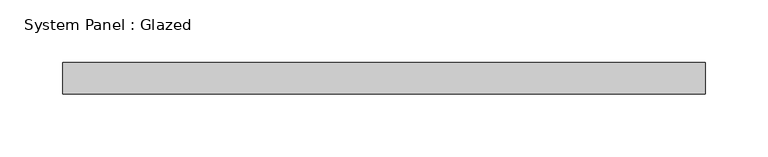
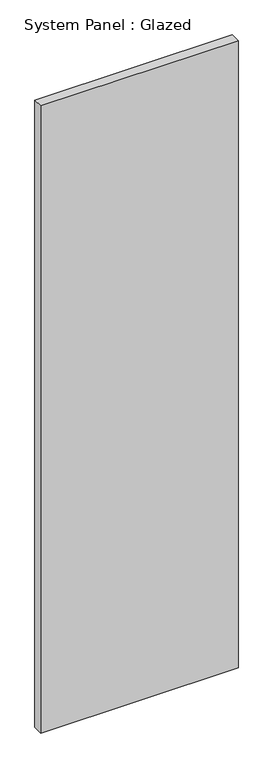
"""IFC4 building model written with IfcOpenShell, lengths in millimetres: plate geometry, System Panel : Glazed."""

from ifc_helpers import new_model, si_unit, origin, origin_with_axes, place, context, project, spatial, polyline, outline, extrude, source, transform, mapped, element, save


def system_panel_glazed_5c6be660(model_context):
    return source(origin(), model_context, "Body", "SweptSolid", [
        extrude(outline(polyline([(257.175, 19.05), (-257.175, 19.05), (-257.175, 44.45), (257.175, 44.45), (257.175, 19.05)])), origin_with_axes(), (0.0, 0.0, 1.0), 1727.2),
    ])


if __name__ == "__main__":
    model = new_model("IFC4")
    model_context = context("Model", 3, world=origin())
    ifc_project = project(units=[si_unit("LENGTHUNIT", "METRE", prefix="MILLI")], contexts=[model_context])
    site = spatial("IfcSite", under=ifc_project)
    building = spatial("IfcBuilding", under=site)
    placement = place(None, origin())
    system_panel_glazed_shape = system_panel_glazed_5c6be660(model_context)
    element("IfcPlate", 1, ObjectType="System Panel : Glazed", at=placement, inside=building, context=model_context, shape_type="MappedRepresentation", body=[
        mapped(system_panel_glazed_shape, transform((0.0, 0.0, 0.0), x_axis=(1.0, 0.0, 0.0), y_axis=(0.0, 1.0, 0.0), z_axis=(0.0, 0.0, 1.0))),
    ])
    save(model, "model.ifc")

# Revit data of these elements
# Type "System Panel : Glazed"
#   Construction Type Id = "GSP4R"
#   Analytic Construction = "1/8 in Pilkington single glazing"
#   Visual Light Transmittance = 0.9
#   Solar Heat Gain Coefficient = 0.86
#   Heat Transfer Coefficient (U) = 1.18115 BTU/(h·ft²·°F)
#   Define Thermal Properties by = 1
# Element 1 (IfcPlate, "System Panel : Glazed")
#   Materials on its faces: "Glass"
# Materials
#   "Glass": class "Glass", colour RGB 0 128 192, transparency 0.75, Description = "Soda Lime Glass", Cost = 0
